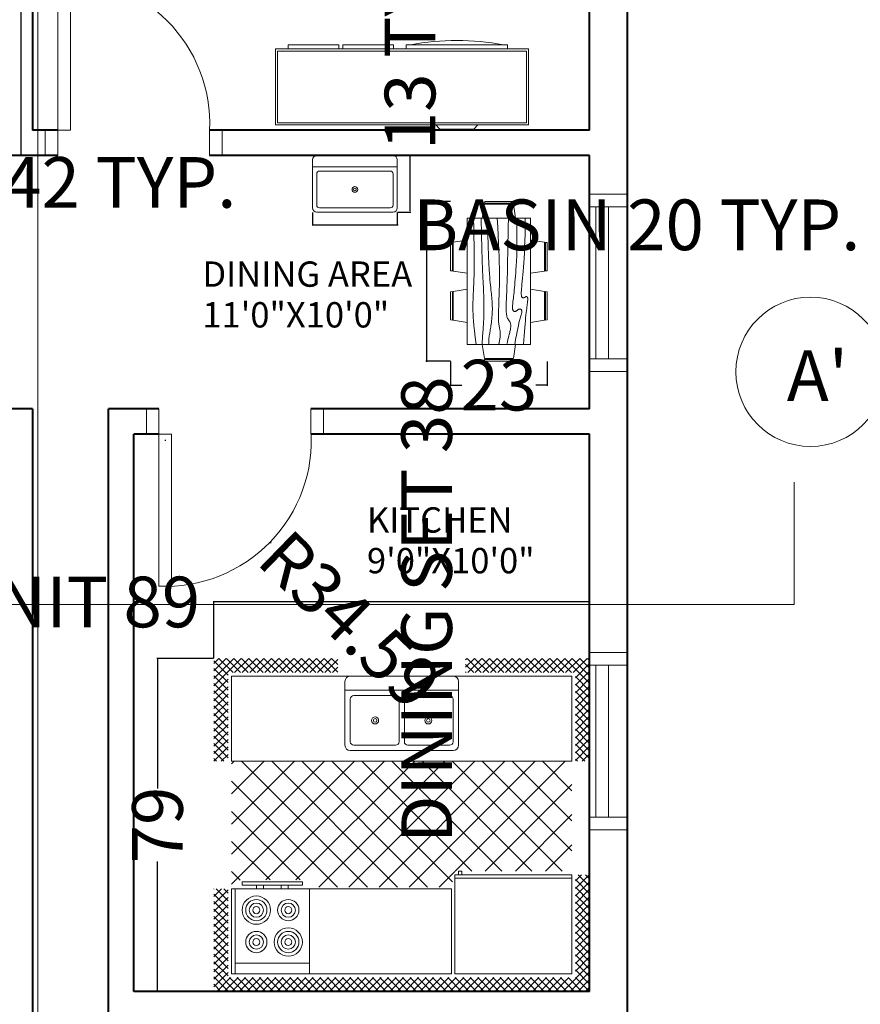
# Model space of a CAD drawing. Units: inches. Extents: x -101 to 786, y 26 to 880.
# Tile 4 of 9: x 180 to 379, y 422 to 655. Entities that reach past the tile are written whole.
import ezdxf

# ---------------------------------------------------------------- set-up
doc = ezdxf.new("R2010")
doc.units = ezdxf.units.IN
doc.header["$MEASUREMENT"] = 0
for name, color, linetype, lineweight in [('A-ANNO-DIMS', 2, 'Continuous', 18), ('A-ANNO-SYMB', 2, 'Continuous', 18), ('A-AREA-IDEN', 7, 'Continuous', 18), ('A-DOOR', 4, 'Continuous', 20), ('A-EQPM', 8, 'Continuous', 13), ('A-FLOR-FIXT', 8, 'Continuous', 18), ('A-FURN', 8, 'Continuous', 13), ('A-GLAZ', 4, 'Continuous', 18), ('A-WALL', 7, 'Continuous', 40)]:
    doc.layers.add(name, color=color, linetype=linetype, lineweight=lineweight)
doc.styles.get("Standard").update_dxf_attribs({"font": 'arial.ttf'})
doc.dimstyles.get("Standard").update_dxf_attribs({"dimtxt": 12, "dimasz": 0.18, "dimexe": 0.18, "dimexo": 0.0625, "dimgap": 0.09, "dimtad": 0, "dimdec": 1, "dimzin": 0, "dimdsep": 46, "dimlunit": 3, "dimtxsty": 'Standard', "dimcen": 0.09, "dimadec": 0, "dimazin": 0, "dimtfac": 1, "dimtdec": 1, "dimtofl": 0, "dimtmove": 0, "dimatfit": 3, "dimfxl": 1, "dimtolj": 1, "dimtzin": 0, "dimarcsym": 0})

# ---------------------------------------------------------------- blocks, each defined once
blk = doc.blocks.new('Kitchen Layout - 7 x 8 ft')
for p, q in [((-5, 81.32), (2.68, 89)), ((-5, 83.44), (0.56, 89)), ((-5, 85.56), (-1.56, 89)), ((-5, 87.68), (-3.68, 89)), ((-1, 84.97), (-5, 88.97)), ((1.09, 85), (-2.91, 89)), ((3.21, 85), (-0.79, 89)), ((0.81, 85), (4.81, 89)), ((5.34, 85), (1.34, 89)), ((2.93, 85), (6.93, 89)), ((7.46, 85), (3.46, 89)), ((5.05, 85), (9.05, 89)), ((9.58, 85), (5.58, 89)), ((7.17, 85), (11.17, 89)), ((11.7, 85), (7.7, 89)), ((9.29, 85), (13.29, 89)), ((13.82, 85), (9.82, 89)), ((11.41, 85), (15.41, 89)), ((15.94, 85), (11.94, 89)), ((13.53, 85), (17.53, 89)), ((18.06, 85), (14.06, 89)), ((15.65, 85), (19.65, 89)), ((20.18, 85), (16.18, 89)), ((17.78, 85), (21.78, 89)), ((22.31, 85), (18.31, 89)), ((19.9, 85), (23.9, 89)), ((24.43, 85), (20.43, 89)), ((22.02, 85), (26.02, 89)), ((26.55, 85), (22.55, 89)), ((24.14, 85), (28.14, 89)), ((28.67, 85), (24.67, 89)), ((26.26, 85), (30.26, 89)), ((30.79, 85), (26.79, 89)), ((28.38, 85), (32.38, 89)), ((32.91, 85), (28.91, 89)), ((30.5, 85), (34.5, 89)), ((35.03, 85), (31.03, 89)), ((32.63, 85), (36.63, 89)), ((37.16, 85), (33.16, 89)), ((34.75, 85), (38.75, 89)), ((39.28, 85), (35.28, 89)), ((36.87, 85), (40.87, 89)), ((41.4, 85), (37.4, 89)), ((38.99, 85), (42.99, 89)), ((43.52, 85), (39.52, 89)), ((41.11, 85), (45.11, 89)), ((45.64, 85), (41.64, 89)), ((43.23, 85), (47.23, 89)), ((47.76, 85), (43.76, 89)), ((45.35, 85), (49.35, 89)), ((49.88, 85), (45.88, 89)), ((47.47, 85), (51.47, 89)), ((52, 85), (48, 89)), ((49.6, 85), (53.6, 89)), ((54.13, 85), (50.13, 89)), ((51.72, 85), (55.72, 89)), ((56.25, 85), (52.25, 89)), ((53.84, 85), (57.84, 89)), ((58.37, 85), (54.37, 89)), ((55.96, 85), (59.96, 89)), ((60.49, 85), (56.49, 89)), ((58.08, 85), (62.08, 89)), ((62.61, 85), (58.61, 89)), ((60.2, 85), (64.2, 89)), ((64.73, 85), (60.73, 89)), ((62.32, 85), (66.32, 89)), ((66.85, 85), (62.85, 89)), ((64.45, 85), (68.45, 89)), ((68.97, 85), (64.97, 89)), ((66.57, 85), (70.57, 89)), ((71.1, 85), (67.1, 89)), ((68.69, 85), (72.69, 89)), ((73.22, 85), (69.22, 89)), ((70.81, 85), (74.81, 89)), ((75.34, 85), (71.34, 89)), ((72.93, 85), (76.93, 89)), ((77.46, 85), (73.46, 89)), ((75.05, 85), (79.05, 89)), ((79.58, 85), (75.58, 89)), ((77.17, 85), (81.17, 89)), ((81.7, 85), (77.7, 89)), ((79.29, 85), (83.29, 89)), ((83.82, 85), (79.82, 89)), ((81.42, 85), (85.42, 89)), ((85.95, 85), (81.95, 89)), ((83.54, 85), (87.54, 89)), ((88.07, 85), (84.07, 89)), ((85.66, 85), (89.66, 89)), ((90.19, 85), (86.19, 89)), ((87.78, 85), (91.78, 89)), ((92.31, 85), (88.31, 89)), ((89.9, 85), (93.9, 89)), ((94.43, 85), (90.43, 89)), ((92.02, 85), (96.02, 89)), ((96.55, 85), (92.55, 89)), ((94.14, 85), (98.14, 89)), ((101, 82.67), (94.67, 89)), ((96.27, 85), (100.27, 89)), ((101, 84.79), (96.79, 89)), ((101, 86.92), (98.92, 89)), ((-1, 82.85), (-5, 86.85)), ((97, 83.61), (101, 87.61)), ((-1, 80.73), (-5, 84.73)), ((34, 84), (96, 84)), ((34, 60), (34, 84)), ((96, 84), (96, 60)), ((97, 81.49), (101, 85.49)), ((101, 80.55), (97, 84.55)), ((97, 79.37), (101, 83.37)), ((-5, 79.19), (-1, 83.19)), ((-1, 78.61), (-5, 82.61)), ((-5, 77.07), (-1, 81.07)), ((74, 81), (95, 81)), ((101, 78.43), (97, 82.43)), ((97, 77.25), (101, 81.25)), ((-1, 76.49), (-5, 80.49)), ((-5, 74.95), (-1, 78.95)), ((-1, 74.36), (-5, 78.36)), ((101, 76.31), (97, 80.31)), ((97, 75.13), (101, 79.13)), ((101, 74.19), (97, 78.19)), ((-5, 72.83), (-1, 76.83)), ((-1, 72.24), (-5, 76.24)), ((97, 73.01), (101, 77.01)), ((101, 72.07), (97, 76.07)), ((-5, 70.71), (-1, 74.71)), ((-1, 70.12), (-5, 74.12)), ((-5, 68.59), (-1, 72.59)), ((97, 70.89), (101, 74.89)), ((101, 69.95), (97, 73.95)), ((97, 68.76), (101, 72.76)), ((-1, 68), (-5, 72)), ((-5, 66.47), (-1, 70.47)), ((-1, 65.88), (-5, 69.88)), ((101, 67.82), (97, 71.82)), ((97, 66.64), (101, 70.64)), ((101, 65.7), (97, 69.7)), ((-5, 64.35), (-1, 68.35)), ((-1, 63.76), (-5, 67.76)), ((97, 64.52), (101, 68.52)), ((101, 63.58), (97, 67.58)), ((-5, 62.22), (-1, 66.22)), ((-1, 61.64), (-5, 65.64)), ((-5, 60.1), (-1, 64.1)), ((97, 62.4), (101, 66.4)), ((101, 61.46), (97, 65.46)), ((97, 60.28), (101, 64.28)), ((-1, 59.52), (-5, 63.52)), ((-5, 57.98), (-1, 61.98)), ((-1, 57.39), (-5, 61.39)), ((100.34, 60), (97, 63.34)), ((98.22, 60), (97, 61.22)), ((98.84, 60), (101, 62.16)), ((-1.73, 56), (-5, 59.27)), ((-4.86, 56), (-1, 59.86)), ((10.4, 24), (45.9, 59.5)), ((18.88, 24), (54.38, 59.5)), ((27.37, 24), (62.87, 59.5)), ((33.03, 55.11), (37.41, 59.5)), ((96, 60), (34, 60)), ((35.85, 24), (71.35, 59.5)), ((76.2, 24), (40.7, 59.5)), ((84.68, 24), (49.18, 59.5)), ((93.17, 24), (57.67, 59.5)), ((61.31, 24), (96, 58.69)), ((96, 29.65), (66.15, 59.5)), ((80, 60), (80, 59)), ((82, 59), (82, 60)), ((87, 59), (87, 60)), ((89, 60), (89, 59)), ((100.96, 60), (101, 60.04)), ((-3.85, 56), (-5, 57.15)), ((-2.74, 56), (-1, 57.74)), ((0, 57), (33, 57)), ((31, 55), (31, 56)), ((32, 56), (32, 55)), ((67.71, 24), (33.68, 58.04)), ((44.34, 24), (77.84, 57.5)), ((52.82, 24), (86.32, 57.5)), ((96, 38.14), (76.64, 57.5)), ((96, 46.63), (85.13, 57.5)), ((96, 55.11), (93.57, 57.54)), ((0, 30.57), (24.43, 55)), ((0, 39.06), (15.94, 55)), ((0, 47.54), (7.46, 55)), ((1.91, 24), (32.91, 55)), ((33.77, 24), (2.77, 55)), ((42.26, 24), (11.26, 55)), ((50.74, 24), (19.74, 55)), ((59.23, 24), (28.23, 55)), ((32, 55), (31, 55)), ((69.79, 24), (96, 50.21)), ((25.29, 24), (0, 49.29)), ((78.28, 24), (96, 41.72)), ((16.8, 24), (0, 40.8)), ((8.32, 24), (0, 32.32)), ((86.76, 24), (96, 33.24)), ((-5, 21.92), (-2.92, 24)), ((-5, 19.8), (-1, 23.8)), ((-1, 19.21), (-5, 23.21)), ((-1, 21.33), (-3.67, 24)), ((-1, 23.45), (-1.55, 24)), ((0, 24), (96, 24)), ((0, 0), (0, 24)), ((95.25, 24), (96, 24.75)), ((96, 24), (96, 0)), ((97, 22.1), (98.9, 24)), ((97, 19.97), (101, 23.97)), ((101, 19.03), (97, 23.03)), ((101, 21.16), (98.16, 24)), ((101, 23.28), (100.28, 24)), ((-5, 17.68), (-1, 21.68)), ((-1, 17.09), (-5, 21.09)), ((-5, 15.55), (-1, 19.55)), ((97, 17.85), (101, 21.85)), ((101, 16.91), (97, 20.91)), ((97, 15.73), (101, 19.73)), ((-1, 14.97), (-5, 18.97)), ((-5, 13.43), (-1, 17.43)), ((-1, 12.85), (-5, 16.85)), ((47.25, 6.5), (47.25, 18.5)), ((48.75, 18.5), (48.75, 6.5)), ((101, 14.79), (97, 18.79)), ((97, 13.61), (101, 17.61)), ((101, 12.67), (97, 16.67)), ((-5, 11.31), (-1, 15.31)), ((-1, 10.73), (-5, 14.73)), ((97, 11.49), (101, 15.49)), ((101, 10.55), (97, 14.55)), ((-5, 9.19), (-1, 13.19)), ((-1, 8.6), (-5, 12.6)), ((97, 9.37), (101, 13.37)), ((101, 8.43), (97, 12.43)), ((97, 7.25), (101, 11.25)), ((-5, 7.07), (-1, 11.07)), ((-1, 6.48), (-5, 10.48)), ((-5, 4.95), (-1, 8.95)), ((-1, 4.36), (-5, 8.36)), ((101, 6.31), (97, 10.31)), ((97, 5.12), (101, 9.12)), ((-5, 2.83), (-1, 6.83)), ((-1, 2.24), (-5, 6.24)), ((101, 4.18), (97, 8.18)), ((97, 3), (101, 7)), ((101, 2.06), (97, 6.06)), ((-5, 0.71), (-1, 4.71)), ((-1, 0.12), (-5, 4.12)), ((64, 4), (32, 4)), ((97, 0.88), (101, 4.88)), ((101, -0.06), (97, 3.94)), ((-5, -1.42), (-1, 2.58)), ((2, -5), (-5, 2)), ((-5, -3.54), (-1, 0.46)), ((96, 0), (0, 0)), ((93.24, -5), (101, 2.76)), ((95.36, -5), (101, 0.64)), ((101, -2.18), (97, 1.82)), ((-0.12, -5), (-5, -0.12)), ((-2.25, -5), (-5, -2.25)), ((-4.34, -5), (-0.34, -1)), ((-2.22, -5), (1.78, -1)), ((-0.1, -5), (3.9, -1)), ((4.12, -5), (0.12, -1)), ((2.02, -5), (6.02, -1)), ((6.24, -5), (2.24, -1)), ((4.14, -5), (8.14, -1)), ((8.36, -5), (4.36, -1)), ((6.27, -5), (10.27, -1)), ((10.48, -5), (6.48, -1)), ((8.39, -5), (12.39, -1)), ((12.6, -5), (8.6, -1)), ((10.51, -5), (14.51, -1)), ((14.73, -5), (10.73, -1)), ((12.63, -5), (16.63, -1)), ((16.85, -5), (12.85, -1)), ((14.75, -5), (18.75, -1)), ((18.97, -5), (14.97, -1)), ((16.87, -5), (20.87, -1)), ((21.09, -5), (17.09, -1)), ((18.99, -5), (22.99, -1)), ((23.21, -5), (19.21, -1)), ((21.11, -5), (25.11, -1)), ((25.33, -5), (21.33, -1)), ((23.24, -5), (27.24, -1)), ((27.45, -5), (23.45, -1)), ((25.36, -5), (29.36, -1)), ((29.57, -5), (25.57, -1)), ((27.48, -5), (30, -2.48)), ((30, -3.3), (27.7, -1)), ((30, -1.18), (29.82, -1)), ((66, -2.54), (67.54, -1)), ((66, -4.66), (69.66, -1)), ((69.88, -5), (66, -1.12)), ((67.78, -5), (71.78, -1)), ((72, -5), (68, -1)), ((69.9, -5), (73.9, -1)), ((74.12, -5), (70.12, -1)), ((72.03, -5), (76.03, -1)), ((76.24, -5), (72.24, -1)), ((74.15, -5), (78.15, -1)), ((78.36, -5), (74.36, -1)), ((76.27, -5), (80.27, -1)), ((80.49, -5), (76.49, -1)), ((78.39, -5), (82.39, -1)), ((82.61, -5), (78.61, -1)), ((80.51, -5), (84.51, -1)), ((84.73, -5), (80.73, -1)), ((82.63, -5), (86.63, -1)), ((86.85, -5), (82.85, -1)), ((84.75, -5), (88.75, -1)), ((88.97, -5), (84.97, -1)), ((86.88, -5), (90.88, -1)), ((91.09, -5), (87.09, -1)), ((89, -5), (93, -1)), ((93.21, -5), (89.21, -1)), ((91.12, -5), (95.12, -1)), ((95.34, -5), (91.34, -1)), ((97.46, -5), (93.46, -1)), ((99.58, -5), (95.58, -1)), ((101, -4.3), (97, -0.3)), ((97.48, -5), (101, -1.48)), ((-4.37, -5), (-5, -4.37)), ((29.6, -5), (30, -4.6)), ((67.76, -5), (66, -3.24)), ((99.6, -5), (101, -3.6))]:
    blk.add_line(p, q)
for points in [[(0, 56), (0, 84), (33, 84), (33, 56)], [(74, 60), (74, 84), (95, 84), (95, 60)], [(76, 58), (76, 59), (93, 59), (93, 58)]]:
    blk.add_lwpolyline(points, close=True)
for points in [[(32, 1.5), (32, 19.5)], [(33.5, 21), (62.5, 21)], [(34.5, 19.5), (46.25, 19.5)], [(49.75, 19.5), (61.5, 19.5)], [(64, 19.5), (64, 1.5)], [(33.5, 6.5), (33.5, 18.5)], [(62.5, 18.5), (62.5, 6.5)], [(46.25, 5.5), (34.5, 5.5)], [(61.5, 5.5), (49.75, 5.5)], [(62.5, 0), (33.5, 0)]]:
    blk.add_lwpolyline(points)
for centre, radius in [((80, 75), 4), ((80, 75), 3), ((89, 75), 3), ((80, 75), 2), ((80, 75), 1), ((89, 75), 2), ((89, 75), 1), ((89, 66), 4), ((80, 66), 3), ((80, 66), 2), ((80, 66), 1), ((89, 66), 3), ((89, 66), 2), ((89, 66), 1), ((40.5, 12.5), 1), ((40.5, 12.5), 0.5), ((55.5, 12.5), 1), ((55.5, 12.5), 0.5)]:
    blk.add_circle(centre, radius)
for centre, radius, start, end in [((33.5, 19.5), 1.5, 90, 180), ((34.5, 18.5), 1, 90, 180), ((46.25, 18.5), 1, 0, 90), ((49.75, 18.5), 1, 90, 180), ((61.5, 18.5), 1, 0, 90), ((62.5, 19.5), 1.5, 0, 90), ((34.5, 6.5), 1, 180, 270), ((46.25, 6.5), 1, 270, 0), ((49.75, 6.5), 1, 180, 270), ((61.5, 6.5), 1, 270, 0), ((33.5, 1.5), 1.5, 180, 270), ((62.5, 1.5), 1.5, 270, 0)]:
    blk.add_arc(centre, radius, start, end)
blk = doc.blocks.new('Dining Set - 36 x 72 in.')
for p, q in [((-22.2343, 26.00059), (-23.4847, 17.99762)), ((-22.2304, 26), (-5.7608, 26)), ((-22, 27.5), (-22.1562, 26.50042)), ((-5.8416, 26.5), (-22.1534, 26.5)), ((-22, 27.5), (-6, 27.5)), ((-5.8437, 26.49966), (-6, 27.5)), ((-4.5152, 17.99762), (-5.7655, 25.99926)), ((5.7657, 26.00059), (4.5153, 17.99762)), ((5.7696, 26), (22.2392, 26)), ((6, 27.5), (5.8438, 26.50042)), ((22.1584, 26.5), (5.8466, 26.5)), ((6, 27.5), (22, 27.5)), ((22.1563, 26.49966), (22, 27.5)), ((23.4848, 17.99762), (22.2345, 25.99926)), ((36, 18), (-36, 18)), ((-36, 18), (-36, -18)), ((36, -18), (36, 18)), ((-45.5, 8), (-44.5004, 8.15617)), ((-45.5, 8), (-45.5, -8)), ((-44.5, -8.15843), (-44.5, 8.15338)), ((-44.0006, 8.23428), (-35.9976, 9.48474)), ((-44, 8.23041), (-44, -8.23915)), ((44.0006, 8.23428), (35.9976, 9.48474)), ((44, 8.23041), (44, -8.23915)), ((44.5, -8.15843), (44.5, 8.15338)), ((45.5, 8), (44.5005, 8.15617)), ((45.5, 8), (45.5, -8)), ((-44.4997, -8.15631), (-45.5, -8)), ((-35.9976, -9.48476), (-43.9993, -8.2345)), ((35.9976, -9.48476), (43.9993, -8.2345)), ((44.4997, -8.15631), (45.5, -8)), ((-36, -18), (36, -18)), ((-22.2343, -26.0006), (-23.4847, -17.99762)), ((-4.5152, -17.99762), (-5.7655, -25.99928)), ((5.7657, -26.0006), (4.5153, -17.99762)), ((23.4848, -17.99762), (22.2345, -25.99928)), ((-22.2304, -26), (-5.7608, -26)), ((-22, -27.5), (-22.1562, -26.50044)), ((-5.8416, -26.5), (-22.1534, -26.5)), ((-22, -27.5), (-6, -27.5)), ((-5.8437, -26.49967), (-6, -27.5)), ((5.7696, -26), (22.2392, -26)), ((6, -27.5), (5.8438, -26.50044)), ((22.1584, -26.5), (5.8466, -26.5)), ((6, -27.5), (22, -27.5)), ((22.1563, -26.49967), (22, -27.5))]:
    blk.add_line(p, q)
for points in [[(-36, 15), (-31.1772, 14.97754), (-26.8079, 14.91406), (-22.8538, 14.81543), (-19.276, 14.6875), (-16.0362, 14.53613), (-13.0957, 14.36718), (-10.4159, 14.18652), (-7.9583, 14), (-5.6904, 13.81315), (-3.6035, 13.63021), (-1.6954, 13.45508), (0.0365, 13.29166), (1.5945, 13.14388), (2.9811, 13.01562), (4.1988, 12.9108), (5.25, 12.83333), (6.1393, 12.78613), (6.8802, 12.76823), (7.4883, 12.77767), (7.9792, 12.8125), (8.3685, 12.87077), (8.6719, 12.95052), (8.9049, 13.0498), (9.0833, 13.16666), (9.2205, 13.29899), (9.3216, 13.44401), (9.3895, 13.59879), (9.4271, 13.76041), (9.4373, 13.92594), (9.4232, 14.09245), (9.3875, 14.257), (9.3333, 14.41666), (9.2638, 14.56917), (9.1836, 14.71484), (9.0975, 14.85465), (9.0104, 14.98958), (8.9272, 15.1206), (8.8529, 15.2487), (8.7922, 15.37483), (8.75, 15.5), (8.7305, 15.62467), (8.7344, 15.74739), (8.7617, 15.86621), (8.8125, 15.97916), (8.8867, 16.08431), (8.9844, 16.17968), (9.1055, 16.26334), (9.25, 16.33333), (9.4189, 16.38802), (9.6172, 16.42708), (9.8506, 16.45052), (10.125, 16.45833), (10.4463, 16.45052), (10.8203, 16.42708), (11.2529, 16.38802), (11.75, 16.33333), (12.3184, 16.26318), (12.9694, 16.17838), (13.7151, 16.07991), (14.5677, 15.96875), (15.5395, 15.84586), (16.6426, 15.71224), (17.8893, 15.56884), (19.2917, 15.41666), (20.859, 15.25667), (22.5879, 15.08984), (24.4721, 14.91715), (26.5052, 14.73958), (28.6809, 14.5581), (30.9929, 14.3737), (33.4347, 14.18733), (36, 14)], [(-36, 10), (-28.9766, 10.14274), (-23.1725, 10.20442), (-18.4241, 10.19775), (-14.5677, 10.13541), (-11.4399, 10.03011), (-8.877, 9.89453), (-6.7154, 9.74137), (-4.7917, 9.58333), (-2.9698, 9.43082), (-1.2246, 9.28515), (0.4415, 9.14534), (2.026, 9.01041), (3.5266, 8.87939), (4.9408, 8.7513), (6.266, 8.62516), (7.5, 8.5), (8.6411, 8.37549), (9.6914, 8.2539), (10.6538, 8.13818), (11.5312, 8.03125), (12.3267, 7.93603), (13.043, 7.85547), (13.6831, 7.79248), (14.25, 7.75), (14.7471, 7.7303), (15.1797, 7.73307), (15.5537, 7.75732), (15.875, 7.80208), (16.1494, 7.86637), (16.3828, 7.94922), (16.5811, 8.04964), (16.75, 8.16666), (16.8944, 8.29915), (17.0143, 8.44531), (17.1089, 8.60319), (17.1771, 8.77083), (17.218, 8.94629), (17.2305, 9.1276), (17.2137, 9.31282), (17.1667, 9.5), (17.0895, 9.6875), (16.987, 9.875), (16.8649, 10.0625), (16.7292, 10.25), (16.5856, 10.4375), (16.4401, 10.625), (16.2985, 10.8125), (16.1667, 11), (16.05, 11.18733), (15.9518, 11.3737), (15.8752, 11.5581), (15.8229, 11.73958), (15.798, 11.91715), (15.8034, 12.08984), (15.842, 12.25667), (15.9167, 12.41666), (16.0295, 12.56836), (16.1784, 12.70833), (16.3605, 12.83268), (16.5729, 12.9375), (16.8127, 13.01888), (17.0768, 13.07291), (17.3625, 13.0957), (17.6667, 13.08333), (17.9894, 13.03312), (18.3418, 12.94726), (18.7382, 12.82918), (19.1927, 12.68229), (19.7195, 12.51001), (20.3327, 12.31575), (21.0465, 12.10294), (21.875, 11.875), (22.8357, 11.63354), (23.959, 11.37304), (25.2786, 11.08618), (26.8282, 10.76562), (28.6414, 10.40405), (30.752, 9.99414), (33.1936, 9.52856), (36, 9)], [(-36, 5.5), (-30.7157, 5.3348), (-26.069, 5.20963), (-21.9946, 5.11767), (-18.4271, 5.05208), (-15.3009, 5.00602), (-12.5508, 4.97265), (-10.1112, 4.94515), (-7.9167, 4.91666), (-5.909, 4.88167), (-4.0586, 4.83984), (-2.3429, 4.79215), (-0.7396, 4.73958), (0.7739, 4.6831), (2.22, 4.6237), (3.6213, 4.56233), (5, 4.5), (6.373, 4.43782), (7.7344, 4.3776), (9.0723, 4.32129), (10.375, 4.27083), (11.6309, 4.22819), (12.8281, 4.19531), (13.9551, 4.17415), (15, 4.16666), (15.954, 4.17448), (16.819, 4.19791), (17.6001, 4.23698), (18.3021, 4.29166), (18.9299, 4.36198), (19.4883, 4.44791), (19.9823, 4.54948), (20.4167, 4.66666), (20.7969, 4.79899), (21.1302, 4.94401), (21.4245, 5.09879), (21.6875, 5.26041), (21.9271, 5.42594), (22.1511, 5.59245), (22.3672, 5.757), (22.5834, 5.91666), (22.8065, 6.06868), (23.0404, 6.21093), (23.2879, 6.34147), (23.5521, 6.45833), (23.8358, 6.55957), (24.142, 6.64323), (24.4735, 6.70735), (24.8334, 6.75), (25.2235, 6.76969), (25.642, 6.76692), (26.0858, 6.74267), (26.5521, 6.69791), (27.0379, 6.63362), (27.5404, 6.55078), (28.0565, 6.45036), (28.5834, 6.33333), (29.1242, 6.19987), (29.7071, 6.04687), (30.3661, 5.87044), (31.1354, 5.66666), (32.0493, 5.43164), (33.142, 5.16146), (34.4475, 4.85221), (36, 4.5)], [(-36, -1), (-30.7915, -0.6591), (-26.0195, -0.38216), (-21.6519, -0.16284), (-17.6563, 0.00521), (-14.0005, 0.12833), (-10.6523, 0.21289), (-7.5796, 0.26522), (-4.75, 0.29166), (-2.134, 0.29793), (0.2878, 0.28711), (2.5317, 0.26163), (4.6146, 0.22396), (6.5529, 0.17651), (8.3633, 0.12174), (10.0623, 0.06209), (11.6667, 0), (13.1899, -0.06201), (14.6341, -0.1211), (15.9982, -0.17432), (17.2813, -0.21875), (18.4823, -0.25147), (19.6003, -0.26953), (20.6343, -0.27002), (21.5834, -0.25), (22.4481, -0.20768), (23.2357, -0.14584), (23.9549, -0.06836), (24.6146, 0.02083), (25.2235, 0.11784), (25.7904, 0.21875), (26.3241, 0.31966), (26.8334, 0.41666), (27.3265, 0.50618), (27.8099, 0.58593), (28.2894, 0.65397), (28.7709, 0.70833), (29.2601, 0.74707), (29.763, 0.76823), (30.2855, 0.76985), (30.8334, 0.75), (31.4088, 0.70784), (31.9994, 0.64713), (32.589, 0.57275), (33.1615, 0.48958), (33.7008, 0.4025), (34.1908, 0.3164), (34.6153, 0.23616), (34.9584, 0.16666), (35.2099, 0.11165), (35.3848, 0.07031), (35.504, 0.04069), (35.5886, 0.02083), (35.6594, 0.00879), (35.7377, 0.0026), (35.8442, 0.00032), (36, 0)], [(-36, -6.5), (-27.1843, -6.31267), (-20.084, -6.1263), (-14.469, -5.9419), (-10.1094, -5.76042), (-6.7752, -5.58285), (-4.2363, -5.41016), (-2.2629, -5.24333), (-0.625, -5.08334), (0.8708, -4.93099), (2.2715, -4.78646), (3.5872, -4.64974), (4.8281, -4.52084), (6.0046, -4.39974), (7.127, -4.28646), (8.2053, -4.18099), (9.25, -4.08334), (10.2705, -3.99382), (11.2734, -3.91407), (12.2647, -3.84603), (13.25, -3.79167), (14.2354, -3.75293), (15.2266, -3.73177), (16.2295, -3.73015), (17.25, -3.75), (18.2912, -3.79248), (19.3451, -3.85547), (20.4009, -3.93604), (21.4479, -4.03125), (22.4754, -4.13819), (23.4727, -4.25391), (24.4289, -4.37549), (25.3334, -4.5), (26.1785, -4.62492), (26.9694, -4.74935), (27.7145, -4.87281), (28.4219, -4.99479), (29.1, -5.11483), (29.7572, -5.23242), (30.4016, -5.34709), (31.0417, -5.45834), (31.6837, -5.56437), (32.3262, -5.65821), (32.9658, -5.73153), (33.599, -5.77604), (34.2224, -5.78345), (34.8327, -5.74545), (35.4264, -5.65373), (36, -5.5)], [(-36, -10), (-26.4022, -9.81299), (-18.4675, -9.62891), (-11.9839, -9.45069), (-6.7396, -9.28125), (-2.5226, -9.12354), (0.8789, -8.98047), (3.6769, -8.85498), (6.0833, -8.75), (8.2767, -8.66765), (10.3021, -8.60677), (12.1712, -8.56543), (13.8958, -8.54167), (15.4876, -8.53353), (16.9583, -8.53907), (18.3197, -8.55632), (19.5834, -8.58334), (20.7616, -8.61841), (21.8685, -8.66081), (22.9188, -8.71004), (23.9271, -8.76563), (24.9081, -8.82707), (25.8763, -8.89388), (26.8465, -8.96558), (27.8334, -9.04167), (28.8474, -9.12118), (29.8828, -9.20117), (30.93, -9.27824), (31.9792, -9.34896), (33.0205, -9.40991), (34.0443, -9.45768), (35.0407, -9.48885), (36, -9.5)], [(-36, -14.5), (-30.0881, -14.33513), (-25.0332, -14.21224), (-20.7312, -14.12647), (-17.0781, -14.07292), (-13.97, -14.04671), (-11.3027, -14.04297), (-8.9724, -14.05681), (-6.875, -14.08334), (-4.9224, -14.11833), (-3.0905, -14.16016), (-1.3709, -14.20785), (0.2448, -14.26042), (1.7647, -14.3169), (3.1973, -14.3763), (4.5507, -14.43767), (5.8333, -14.5), (7.0554, -14.5621), (8.235, -14.62175), (9.3922, -14.67652), (10.5469, -14.72396), (11.7192, -14.76164), (12.929, -14.78711), (14.1965, -14.79794), (15.5417, -14.79167), (16.9933, -14.76424), (18.6152, -14.70508), (20.4804, -14.60197), (22.6615, -14.44271), (25.2312, -14.21509), (28.2624, -13.9069), (31.8277, -13.50594), (36, -13)]]:
    blk.add_lwpolyline(points)
blk = doc.blocks.new('Sink-single - 30 in top')
blk.add_line((-15, -3.999996), (15, -3.999996))
for points in [[(-13.5, 0), (13.5, 0)], [(-15, -18.499996), (-15, -1.5)], [(15, -1.5), (15, -18.499996)], [(-13.5, -17.499996), (-13.5, -6.499996)], [(-12.5, -5.499996), (12.5, -5.499996)], [(13.5, -6.499996), (13.5, -17.499996)], [(13.5, -19.999996), (-13.5, -19.999996)], [(12.5, -18.499996), (-12.5, -18.499996)]]:
    blk.add_lwpolyline(points)
for radius in [1, 0.5]:
    blk.add_circle((0, -11.999996), radius)
for centre, radius, start, end in [((-13.5, -1.5), 1.5, 90, 180), ((13.5, -1.5), 1.5, 0, 90), ((-12.5, -6.499996), 1, 90, 180), ((12.5, -6.499996), 1, 0, 90), ((-13.5, -18.499996), 1.5, 180, 270), ((-12.5, -17.499996), 1, 180, 270), ((12.5, -17.499996), 1, 270, 0), ((13.5, -18.499996), 1.5, 270, 0)]:
    blk.add_arc(centre, radius, start, end)
blk = doc.blocks.new('Entertainment Center')
for p, q in [((-4, 0), (-5, -1)), ((4, 0), (-4, 0)), ((5, -1), (4, 0)), ((-17, -19), (-17, -1)), ((-17, -1), (43, -1)), ((-16.5, -18.5), (-16.5, -1.5)), ((-16.5, -1.5), (42.5, -1.5)), ((42.5, -1.5), (42.5, -18.5)), ((43, -1), (43, -19)), ((42.5, -18.5), (-16.5, -18.5)), ((43, -19), (-17, -19)), ((-12, -20), (-12, -19)), ((12, -20), (-12, -20)), ((12, -19), (12, -20)), ((15, -20), (15, -19)), ((27, -20), (15, -20)), ((27, -19), (27, -20)), ((28, -20), (28, -19)), ((40, -20), (28, -20)), ((40, -19), (40, -20))]:
    blk.add_line(p, q)
blk.add_arc((0, 40), 61, 259.6111, 280.3889)
blk = doc.blocks.new('DOOR-SINGLE-36')
for p, q in [((-39, 0), (-39, -6)), ((-36, 0), (-36, -6)), ((0, 0), (0, -6)), ((3, 0), (3, -6))]:
    blk.add_line(p, q)
blk.add_lwpolyline([(0, 0), (-3, 0), (-3, 36), (0, 36)], close=True)
blk.add_arc((-1.5, 1.5), 34.53, 87.5104, 182.4896)
blk = doc.blocks.new('WIN-36-WALL9')
for p, q in [((0, 42), (9, 42)), ((0, 39), (9, 39)), ((1.5, 39), (1.5, 3)), ((4.5, 39), (4.5, 3)), ((9, 3), (0, 3)), ((9, 0), (0, 0))]:
    blk.add_line(p, q)
blk = doc.blocks.new('*D35')
at = {"layer": 'A-ANNO-DIMS', "color": 0, "lineweight": -2, "transparency": 16777216}
for p, q in [((173.57, 665.22), (180.05, 665.22)), ((179.87, 665.22), (179.87, 665.4)), ((179.87, 622.98), (179.87, 665.04)), ((173.57, 622.8), (180.05, 622.8))]:
    blk.add_line(p, q, dxfattribs=at)
at = {"layer": 'A-ANNO-DIMS', "color": 0, "transparency": 16777216}
for points in [[(179.84, 665.04), (179.9, 665.04), (179.87, 665.22)], [(179.84, 622.98), (179.9, 622.98), (179.87, 622.8)]]:
    blk.add_solid(points, dxfattribs=at)
at = {"layer": 'Defpoints', "color": 0, "transparency": 16777216}
for p in [(173.51, 665.22), (179.87, 665.22), (173.51, 622.8)]:
    blk.add_point(p, dxfattribs=at)
at = {"layer": 'A-ANNO-DIMS', "color": 0, "transparency": 16777216, "insert": (179.87, 721.88), "char_height": 12, "attachment_point": 5, "rotation": 90}
blk.add_mtext('\\A1;DOOR 42 TYP.', dxfattribs=at)
blk = doc.blocks.new('*D36')
at = {"layer": 'A-ANNO-DIMS', "color": 0, "lineweight": -2, "transparency": 16777216}
for p, q in [((131.51, 622.74), (131.51, 616.26)), ((173.51, 622.74), (173.51, 616.26)), ((131.69, 616.44), (173.33, 616.44)), ((173.51, 616.44), (173.69, 616.44))]:
    blk.add_line(p, q, dxfattribs=at)
at = {"layer": 'A-ANNO-DIMS', "color": 0, "transparency": 16777216}
for points in [[(131.69, 616.47), (131.69, 616.41), (131.51, 616.44)], [(173.33, 616.47), (173.33, 616.41), (173.51, 616.44)]]:
    blk.add_solid(points, dxfattribs=at)
at = {"layer": 'Defpoints', "color": 0, "transparency": 16777216}
for p in [(131.51, 622.8), (173.51, 622.8), (173.51, 616.44)]:
    blk.add_point(p, dxfattribs=at)
at = {"layer": 'A-ANNO-DIMS', "color": 0, "transparency": 16777216, "insert": (203.22, 616.44), "char_height": 12, "attachment_point": 5}
blk.add_mtext('\\A1;42 TYP.', dxfattribs=at)
blk = doc.blocks.new('*D43')
at = {"layer": 'A-ANNO-DIMS', "color": 0, "lineweight": -2, "transparency": 16777216}
for p, q in [((248.86, 609.34), (248.86, 606.21)), ((268.95, 609.34), (268.95, 606.21)), ((249.04, 606.39), (268.77, 606.39)), ((268.95, 606.39), (269.13, 606.39))]:
    blk.add_line(p, q, dxfattribs=at)
at = {"layer": 'A-ANNO-DIMS', "color": 0, "transparency": 16777216}
for points in [[(249.04, 606.42), (249.04, 606.36), (248.86, 606.39)], [(268.77, 606.42), (268.77, 606.36), (268.95, 606.39)]]:
    blk.add_solid(points, dxfattribs=at)
at = {"layer": 'Defpoints', "color": 0, "transparency": 16777216}
for p in [(248.86, 609.41), (268.95, 609.41), (268.95, 606.39)]:
    blk.add_point(p, dxfattribs=at)
at = {"layer": 'A-ANNO-DIMS', "color": 0, "transparency": 16777216, "insert": (325.65, 606.39), "char_height": 12, "attachment_point": 5}
blk.add_mtext('\\A1;BASIN 20 TYP.', dxfattribs=at)
blk = doc.blocks.new('*D44')
at = {"layer": 'A-ANNO-DIMS', "color": 0, "lineweight": -2, "transparency": 16777216}
for p, q in [((269.02, 622.8), (272.15, 622.8)), ((271.97, 622.8), (271.97, 622.98)), ((271.97, 609.59), (271.97, 622.62)), ((269.02, 609.41), (272.15, 609.41))]:
    blk.add_line(p, q, dxfattribs=at)
at = {"layer": 'A-ANNO-DIMS', "color": 0, "transparency": 16777216}
for points in [[(271.94, 622.62), (272, 622.62), (271.97, 622.8)], [(271.94, 609.59), (272, 609.59), (271.97, 609.41)]]:
    blk.add_solid(points, dxfattribs=at)
at = {"layer": 'Defpoints', "color": 0, "transparency": 16777216}
for p in [(268.95, 622.8), (271.97, 622.8), (268.95, 609.41)]:
    blk.add_point(p, dxfattribs=at)
at = {"layer": 'A-ANNO-DIMS', "color": 0, "transparency": 16777216, "insert": (271.97, 651.71), "char_height": 12, "attachment_point": 5, "rotation": 90}
blk.add_mtext('\\A1;13 TYP.', dxfattribs=at)
blk = doc.blocks.new('*D65')
at = {"layer": 'A-ANNO-DIMS', "color": 0, "lineweight": -2, "transparency": 16777216}
for p, q in [((225.49, 517.07), (225.31, 517.07)), ((225.49, 503.78), (225.49, 517.25)), ((314.33, 517.07), (225.67, 517.07)), ((314.51, 503.78), (314.51, 517.25))]:
    blk.add_line(p, q, dxfattribs=at)
at = {"layer": 'A-ANNO-DIMS', "color": 0, "transparency": 16777216}
for points in [[(225.67, 517.1), (225.67, 517.04), (225.49, 517.07)], [(314.33, 517.1), (314.33, 517.04), (314.51, 517.07)]]:
    blk.add_solid(points, dxfattribs=at)
at = {"layer": 'Defpoints', "color": 0, "transparency": 16777216}
for p in [(225.49, 517.07), (225.49, 503.72), (314.51, 503.72)]:
    blk.add_point(p, dxfattribs=at)
at = {"layer": 'A-ANNO-DIMS', "color": 0, "transparency": 16777216, "insert": (155.88, 517.07), "char_height": 12, "attachment_point": 5}
blk.add_mtext('\\A1;KITCHEN UNIT 89', dxfattribs=at)
blk = doc.blocks.new('*D66')
at = {"layer": 'A-ANNO-DIMS', "color": 0, "lineweight": -2, "transparency": 16777216}
for p, q in [((225.43, 503.72), (211.96, 503.72)), ((212.14, 503.54), (212.14, 472.9)), ((212.14, 424.96), (212.14, 455.6)), ((225.43, 424.78), (211.96, 424.78))]:
    blk.add_line(p, q, dxfattribs=at)
at = {"layer": 'A-ANNO-DIMS', "color": 0, "transparency": 16777216}
for points in [[(212.11, 503.54), (212.17, 503.54), (212.14, 503.72)], [(212.11, 424.96), (212.17, 424.96), (212.14, 424.78)]]:
    blk.add_solid(points, dxfattribs=at)
at = {"layer": 'Defpoints', "color": 0, "transparency": 16777216}
for p in [(225.49, 503.72), (212.14, 424.78), (225.49, 424.78)]:
    blk.add_point(p, dxfattribs=at)
at = {"layer": 'A-ANNO-DIMS', "color": 0, "transparency": 16777216, "insert": (212.14, 464.25), "char_height": 12, "attachment_point": 5, "rotation": 90}
blk.add_mtext('\\A1;79', dxfattribs=at)
blk = doc.blocks.new('*D67')
at = {"layer": 'A-ANNO-DIMS', "color": 0, "lineweight": -2, "transparency": 16777216}
for p, q in [((281.52, 611.94), (275.73, 611.94)), ((275.91, 611.76), (275.91, 574.29)), ((281.52, 574.11), (275.73, 574.11)), ((275.91, 574.11), (275.91, 573.93))]:
    blk.add_line(p, q, dxfattribs=at)
at = {"layer": 'A-ANNO-DIMS', "color": 0, "transparency": 16777216}
for points in [[(275.88, 611.76), (275.94, 611.76), (275.91, 611.94)], [(275.88, 574.29), (275.94, 574.29), (275.91, 574.11)]]:
    blk.add_solid(points, dxfattribs=at)
at = {"layer": 'Defpoints', "color": 0, "transparency": 16777216}
for p in [(281.59, 611.94), (275.91, 574.11), (281.59, 574.11)]:
    blk.add_point(p, dxfattribs=at)
at = {"layer": 'A-ANNO-DIMS', "color": 0, "transparency": 16777216, "insert": (275.91, 515.24), "char_height": 12, "attachment_point": 5, "rotation": 90}
blk.add_mtext('\\A1;DINING SET 38', dxfattribs=at)
blk = doc.blocks.new('*D68')
at = {"layer": 'A-ANNO-DIMS', "color": 0, "lineweight": -2, "transparency": 16777216}
for p, q in [((281.59, 574.05), (281.59, 568.25)), ((304.45, 574.05), (304.45, 568.25)), ((281.77, 568.43), (284.23, 568.43)), ((304.27, 568.43), (301.81, 568.43))]:
    blk.add_line(p, q, dxfattribs=at)
at = {"layer": 'A-ANNO-DIMS', "color": 0, "transparency": 16777216}
for points in [[(281.77, 568.46), (281.77, 568.4), (281.59, 568.43)], [(304.27, 568.46), (304.27, 568.4), (304.45, 568.43)]]:
    blk.add_solid(points, dxfattribs=at)
at = {"layer": 'Defpoints', "color": 0, "transparency": 16777216}
for p in [(281.59, 574.11), (304.45, 574.11), (304.45, 568.43)]:
    blk.add_point(p, dxfattribs=at)
at = {"layer": 'A-ANNO-DIMS', "color": 0, "transparency": 16777216, "insert": (293.02, 568.43), "char_height": 12, "attachment_point": 5}
blk.add_mtext('\\A1;23', dxfattribs=at)
blk = doc.blocks.new('*D80')
at = {"layer": 'A-ANNO-DIMS', "color": 0, "lineweight": -2, "transparency": 16777216}
for p, q in [((323.57, 781.8), (424.94, 781.8)), ((424.76, 781.62), (424.76, 472.49)), ((424.76, 122.52), (424.76, 431.66)), ((323.57, 122.34), (424.94, 122.34))]:
    blk.add_line(p, q, dxfattribs=at)
at = {"layer": 'A-ANNO-DIMS', "color": 0, "transparency": 16777216}
for points in [[(424.73, 781.62), (424.79, 781.62), (424.76, 781.8)], [(424.73, 122.52), (424.79, 122.52), (424.76, 122.34)]]:
    blk.add_solid(points, dxfattribs=at)
at = {"layer": 'Defpoints', "color": 0, "transparency": 16777216}
for p in [(323.51, 781.8), (424.76, 781.8), (323.51, 122.34)]:
    blk.add_point(p, dxfattribs=at)
at = {"layer": 'A-ANNO-DIMS', "color": 0, "transparency": 16777216, "insert": (424.76, 452.07), "char_height": 12, "attachment_point": 5, "rotation": 90}
blk.add_mtext('\\A1;659.5', dxfattribs=at)
blk = doc.blocks.new('*D130')
at = {"layer": 'A-ANNO-DIMS', "color": 0, "lineweight": -2, "transparency": 16777216}
for p, q in [((213.92, 555.36), (214.1, 555.36)), ((214.01, 555.27), (214.01, 555.45)), ((239.08, 531.01), (238.95, 531.14))]:
    blk.add_line(p, q, dxfattribs=at)
at = {"layer": 'A-ANNO-DIMS', "color": 0, "transparency": 16777216}
blk.add_solid([(238.97, 531.16), (238.93, 531.12), (238.82, 531.26)], dxfattribs=at)
at = {"layer": 'Defpoints', "color": 0, "transparency": 16777216}
for p in [(214.01, 555.36), (238.82, 531.26)]:
    blk.add_point(p, dxfattribs=at)
at = {"layer": 'A-ANNO-DIMS', "color": 0, "transparency": 16777216, "insert": (257.8, 512.83), "char_height": 12, "attachment_point": 5, "rotation": 315.8375}
blk.add_mtext('\\A1;R34.59', dxfattribs=at)

msp = doc.modelspace()

# ---------------------------------------------------------------- linework, layer by layer
at = {"layer": 'A-ANNO-SYMB'}
for p, q in [((183.8117, 802.4238), (183.8117, 309.6043)), ((362.9319, 516.4544), (362.9319, 545.4735)), ((-40.6288, 516.4544), (362.9319, 516.4544))]:
    msp.add_line(p, q, dxfattribs=at)
msp.add_circle((366.8306, 571.5872), 17.6773, dxfattribs=at)
at = {"layer": 'A-DOOR'}
for p, q in [((209.5071, 556.8033), (209.5071, 562.8033)), ((212.5071, 556.8033), (212.5071, 562.8033)), ((248.5071, 556.8033), (248.5071, 562.8033)), ((251.5071, 556.8033), (251.5071, 562.8033))]:
    msp.add_line(p, q, dxfattribs=at)
msp.add_lwpolyline([(212.5071, 556.8033), (215.5071, 556.8033), (215.5071, 520.8033), (212.5071, 520.8033)], close=True, dxfattribs=at)
msp.add_arc((214.0071, 555.3619), 34.5912, 267.514665, 4.160516, dxfattribs=at)
at = {"layer": 'A-WALL'}
for p, q in [((182.5071, 772.8033), (182.5071, 628.8033)), ((314.5071, 628.8033), (314.5071, 772.8033)), ((188.5071, 628.8033), (182.5071, 628.8033)), ((314.5071, 628.8033), (224.5071, 628.8033)), ((188.5071, 622.8033), (170.5071, 622.8033)), ((314.5071, 622.8033), (224.5071, 622.8033)), ((314.5071, 562.8033), (314.5071, 622.8033)), ((182.5071, 562.8033), (170.5071, 562.8033)), ((182.5071, 562.8033), (182.5071, 418.8033)), ((200.5071, 418.8033), (200.5071, 562.8033)), ((212.5071, 562.8033), (200.5071, 562.8033)), ((314.5071, 562.8033), (248.5071, 562.8033)), ((206.5071, 424.8033), (206.5071, 556.8033)), ((212.5071, 556.8033), (206.5071, 556.8033)), ((314.5071, 556.8033), (248.5071, 556.8033)), ((314.5071, 424.8033), (314.5071, 556.8033)), ((314.5071, 424.8033), (206.5071, 424.8033))]:
    msp.add_line(p, q, dxfattribs=at)
msp.add_lwpolyline([(323.5071, 151.8033), (323.5071, 781.8033), (23.5071, 781.8033), (23.5071, 151.8033)], dxfattribs=at)

# ---------------------------------------------------------------- block references
at = {"layer": 'A-DOOR', "extrusion": (0, 0, -1), "zscale": -1}
msp.add_blockref('DOOR-SINGLE-36', (-188.5071, 628.8033), dxfattribs=at)
at = {"layer": 'A-EQPM', "rotation": 180}
msp.add_blockref('Entertainment Center', (283.0681, 629.0561), dxfattribs=at)
at = {"layer": 'A-FLOR-FIXT', "xscale": 0.669901374782416, "yscale": 0.669901374782416, "zscale": 0.669901374782416}
msp.add_blockref('Sink-single - 30 in top', (258.9063, 622.8033), dxfattribs=at)
at = {"layer": 'A-FLOR-FIXT', "xscale": 0.8397500674456428, "yscale": 0.8397500674456428, "zscale": 0.8397500674456428, "rotation": 180.0000000000001}
msp.add_blockref('Kitchen Layout - 7 x 8 ft', (310.3083, 499.517), dxfattribs=at)
at = {"layer": 'A-FURN', "xscale": 0.4157739377331477, "yscale": 0.4157739377331477, "zscale": 0.4157739377331477, "rotation": 270}
msp.add_blockref('Dining Set - 36 x 72 in.', (293.0193, 593.0273), dxfattribs=at)
at = {"layer": 'A-GLAZ'}
for p in [(314.507, 571.6587), (314.507, 463.082)]:
    msp.add_blockref('WIN-36-WALL9', p, dxfattribs=at)

# ---------------------------------------------------------------- texts
at = {"layer": 'A-ANNO-SYMB'}
msp.add_text("A'", height=12, dxfattribs=at).set_placement((361.2197, 564.663))
at = {"layer": 'A-AREA-IDEN'}
for s, p in [('DINING AREA', (222.7831, 591.7201)), ('11\'0"X10\'0"', (222.7831, 582.0816)), ('KITCHEN', (261.7683, 533.4982)), ('9\'0"X10\'0"', (261.7683, 523.8597))]:
    msp.add_text(s, height=6, dxfattribs=at).set_placement(p)

# ---------------------------------------------------------------- dimensions: what is measured, and where the dimension line sits
at = {"layer": 'A-ANNO-DIMS'}
for base, p1, p2, angle, override, picture, middle in [((424.7579, 781.8033), (323.5071, 122.3446), (323.5071, 781.8033), 90, {"dimdec": 1, "dimlfac": 1, "dimrnd": 0, "dimzin": 0, "dimdsep": 46, "dimlunit": 2}, '*D80', (424.7579, 452.0739)), ((212.1415, 424.7793), (225.4936, 503.7158), (225.4936, 424.7793), 270, {"dimdec": 0, "dimlfac": 1, "dimrnd": 0, "dimzin": 0, "dimdsep": 46, "dimlunit": 2}, '*D66', (212.1415, 464.2475))]:
    dim = msp.add_linear_dim(base=base, p1=p1, p2=p2, angle=angle, dimstyle='Standard', override=override, dxfattribs=at)
    dim.commit()
    dim.dimension.update_dxf_attribs({"geometry": picture, "text_midpoint": middle})
for base, p1, p2, angle, text, picture, middle in [((179.8701, 665.2238), (173.5071, 622.8033), (173.5071, 665.2238), 90, 'DOOR <> TYP.', '*D35', (179.8701, 721.8757)), ((271.9694, 622.8033), (268.9548, 609.4053), (268.9548, 622.8033), 90, '<> TYP.', '*D44', (271.9694, 651.7145)), ((275.9102, 574.1096), (281.5855, 611.945), (281.5855, 574.1096), 270, 'DINING SET <>', '*D67', (275.9102, 515.2352)), ((225.4936, 517.0678), (314.5071, 503.7158), (225.4936, 503.7158), 180, 'KITCHEN UNIT <>', '*D65', (155.8798, 517.0678))]:
    dim = msp.add_linear_dim(base=base, p1=p1, p2=p2, angle=angle, text=text, dimstyle='Standard', override={"dimdec": 0, "dimlfac": 1, "dimrnd": 0, "dimzin": 0, "dimdsep": 46, "dimlunit": 2}, dxfattribs=at)
    dim.commit()
    dim.dimension.update_dxf_attribs({"geometry": picture, "text_midpoint": middle})
for base, p1, p2, text, picture, middle in [((173.5071, 616.4402), (131.5071, 622.8033), (173.5071, 622.8033), '<> TYP.', '*D36', (203.2245, 616.4402)), ((268.9548, 606.3907), (248.8578, 609.4053), (268.9548, 609.4053), 'BASIN <> TYP.', '*D43', (325.6477, 606.3907))]:
    dim = msp.add_linear_dim(base=base, p1=p1, p2=p2, text=text, dimstyle='Standard', override={"dimdec": 0, "dimlfac": 1, "dimrnd": 0, "dimzin": 0, "dimdsep": 46, "dimlunit": 2}, dxfattribs=at)
    dim.commit()
    dim.dimension.update_dxf_attribs({"geometry": picture, "text_midpoint": middle})
dim = msp.add_linear_dim(base=(304.4531, 568.4342), p1=(281.5855, 574.1096), p2=(304.4531, 574.1096), dimstyle='Standard', override={"dimdec": 0, "dimlfac": 1, "dimrnd": 0, "dimzin": 0, "dimdsep": 46, "dimlunit": 2}, dxfattribs=at)
dim.commit()
dim.dimension.update_dxf_attribs({"geometry": '*D68', "text_midpoint": (293.0193, 568.4342)})
dim = msp.add_radius_dim(center=(214.0071, 555.3619), mpoint=(238.8216, 531.2624), dimstyle='Standard', override={"dimdec": 2, "dimlfac": 1, "dimrnd": 0, "dimzin": 0, "dimdsep": 46, "dimlunit": 2}, dxfattribs=at)
dim.commit()
dim.dimension.update_dxf_attribs({"geometry": '*D130', "text_midpoint": (257.7969, 512.8338)})

doc.saveas('drawing.dxf')
